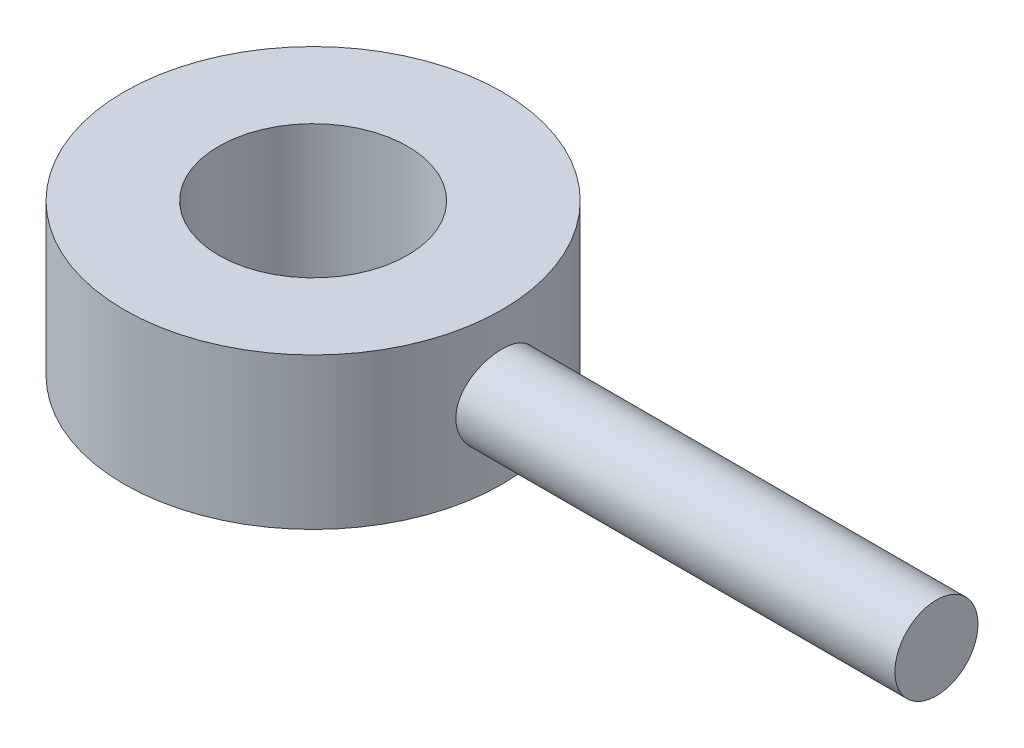
ISO-10303-21;
HEADER;
FILE_DESCRIPTION(('STEP AP214'),'2;1');
FILE_NAME('part.step','',(''),(''),'','','');
FILE_SCHEMA(('AUTOMOTIVE_DESIGN { 1 0 10303 214 1 1 1 1 }'));
ENDSEC;
DATA;
#1=APPLICATION_CONTEXT('core data for automotive mechanical design processes');
#2=APPLICATION_PROTOCOL_DEFINITION('international standard','automotive_design',2000,#1);
#3=PRODUCT_CONTEXT('',#1,'mechanical');
#4=PRODUCT('Part','Part','',(#3));
#5=PRODUCT_RELATED_PRODUCT_CATEGORY('part','',(#4));
#6=PRODUCT_DEFINITION_FORMATION('','',#4);
#7=PRODUCT_DEFINITION_CONTEXT('part definition',#1,'design');
#8=PRODUCT_DEFINITION('design','',#6,#7);
#9=PRODUCT_DEFINITION_SHAPE('','',#8);
#10=(LENGTH_UNIT() NAMED_UNIT(*) SI_UNIT(.MILLI.,.METRE.));
#11=(NAMED_UNIT(*) PLANE_ANGLE_UNIT() SI_UNIT($,.RADIAN.));
#12=(NAMED_UNIT(*) SI_UNIT($,.STERADIAN.) SOLID_ANGLE_UNIT());
#13=UNCERTAINTY_MEASURE_WITH_UNIT(LENGTH_MEASURE(1.E-05),#10,'distance_accuracy_value','');
#14=(GEOMETRIC_REPRESENTATION_CONTEXT(3) GLOBAL_UNCERTAINTY_ASSIGNED_CONTEXT((#13)) GLOBAL_UNIT_ASSIGNED_CONTEXT((#10,
#11,#12)) REPRESENTATION_CONTEXT('',''));
#15=CARTESIAN_POINT('',(0.,0.,0.));
#16=DIRECTION('',(0.,0.,1.));
#17=DIRECTION('',(1.,0.,0.));
#18=AXIS2_PLACEMENT_3D('',#15,#16,#17);
#19=CARTESIAN_POINT('',(0.,4.,0.));
#20=DIRECTION('',(0.,1.,0.));
#21=DIRECTION('',(0.,0.,1.));
#22=AXIS2_PLACEMENT_3D('',#19,#20,#21);
#23=PLANE('',#22);
#24=CARTESIAN_POINT('',(0.,4.,0.));
#25=DIRECTION('',(0.,1.,0.));
#26=DIRECTION('',(0.,0.,1.));
#27=AXIS2_PLACEMENT_3D('',#24,#25,#26);
#28=CIRCLE('',#27,5.);
#29=CARTESIAN_POINT('',(0.,4.,5.));
#30=VERTEX_POINT('',#29);
#31=EDGE_CURVE('E10',#30,#30,#28,.T.);
#32=ORIENTED_EDGE('',*,*,#31,.T.);
#33=EDGE_LOOP('',(#32));
#34=FACE_BOUND('',#33,.T.);
#35=CARTESIAN_POINT('',(0.,4.,0.));
#36=DIRECTION('',(0.,1.,0.));
#37=DIRECTION('',(0.,0.,1.));
#38=AXIS2_PLACEMENT_3D('',#35,#36,#37);
#39=CIRCLE('',#38,2.5);
#40=CARTESIAN_POINT('',(0.,4.,2.5));
#41=VERTEX_POINT('',#40);
#42=EDGE_CURVE('E47',#41,#41,#39,.T.);
#43=ORIENTED_EDGE('',*,*,#42,.F.);
#44=EDGE_LOOP('',(#43));
#45=FACE_BOUND('',#44,.T.);
#46=ADVANCED_FACE('F40',(#34,#45),#23,.T.);
#47=CARTESIAN_POINT('',(0.,0.,0.));
#48=DIRECTION('',(0.,1.,0.));
#49=DIRECTION('',(0.,0.,1.));
#50=AXIS2_PLACEMENT_3D('',#47,#48,#49);
#51=PLANE('',#50);
#52=CARTESIAN_POINT('',(0.,0.,0.));
#53=DIRECTION('',(0.,1.,0.));
#54=DIRECTION('',(0.,0.,1.));
#55=AXIS2_PLACEMENT_3D('',#52,#53,#54);
#56=CIRCLE('',#55,5.);
#57=CARTESIAN_POINT('',(0.,0.,5.));
#58=VERTEX_POINT('',#57);
#59=EDGE_CURVE('E45',#58,#58,#56,.T.);
#60=ORIENTED_EDGE('',*,*,#59,.F.);
#61=EDGE_LOOP('',(#60));
#62=FACE_BOUND('',#61,.T.);
#63=CARTESIAN_POINT('',(0.,0.,0.));
#64=DIRECTION('',(0.,1.,0.));
#65=DIRECTION('',(0.,0.,1.));
#66=AXIS2_PLACEMENT_3D('',#63,#64,#65);
#67=CIRCLE('',#66,2.5);
#68=CARTESIAN_POINT('',(0.,0.,2.5));
#69=VERTEX_POINT('',#68);
#70=EDGE_CURVE('E51',#69,#69,#67,.T.);
#71=ORIENTED_EDGE('',*,*,#70,.T.);
#72=EDGE_LOOP('',(#71));
#73=FACE_BOUND('',#72,.T.);
#74=ADVANCED_FACE('F76',(#62,#73),#51,.F.);
#75=CARTESIAN_POINT('',(0.,4.,0.));
#76=DIRECTION('',(0.,-1.,0.));
#77=DIRECTION('',(0.,0.,-1.));
#78=AXIS2_PLACEMENT_3D('',#75,#76,#77);
#79=CYLINDRICAL_SURFACE('',#78,5.);
#80=CARTESIAN_POINT('',(4.87749935930288,2.,-1.1));
#81=CARTESIAN_POINT('',(4.87750059192786,1.9390201794353,-1.09999791492612));
#82=CARTESIAN_POINT('',(4.87865539644142,1.87801537811326,-1.09491201866376));
#83=CARTESIAN_POINT('',(4.88314122250592,1.75774129032022,-1.07472546298642));
#84=CARTESIAN_POINT('',(4.88647380552498,1.69847328101234,-1.05961761771207));
#85=CARTESIAN_POINT('',(4.89491990534441,1.58342998059707,-1.0198864288525));
#86=CARTESIAN_POINT('',(4.90003145433793,1.52765091028854,-0.995273595944624));
#87=CARTESIAN_POINT('',(4.91145717082736,1.42101230207449,-0.937261257278608));
#88=CARTESIAN_POINT('',(4.91777131651074,1.37015267496603,-0.903861910884835));
#89=CARTESIAN_POINT('',(4.93101133539934,1.27392683949134,-0.828616225712396));
#90=CARTESIAN_POINT('',(4.93794511097895,1.22865694066119,-0.786648093254168));
#91=CARTESIAN_POINT('',(4.95157396934833,1.1457392824436,-0.695719054453303));
#92=CARTESIAN_POINT('',(4.95826903341563,1.10809211983954,-0.646757601115515));
#93=CARTESIAN_POINT('',(4.97075222751559,1.04110713566132,-0.542585501574227));
#94=CARTESIAN_POINT('',(4.97652994590525,1.0118620215218,-0.487313887417924));
#95=CARTESIAN_POINT('',(4.98643815937044,0.963111197150299,-0.372492215823986));
#96=CARTESIAN_POINT('',(4.99056884147107,0.943604381046737,-0.312942645065845));
#97=CARTESIAN_POINT('',(4.99666172270461,0.915187000374263,-0.19225695217033));
#98=CARTESIAN_POINT('',(4.99865724849314,0.906113415539374,-0.131160926699203));
#99=CARTESIAN_POINT('',(5.00037046767797,0.898310289156249,-0.00828344107533812));
#100=CARTESIAN_POINT('',(5.00008842457891,0.899579550986583,0.0534979389590024));
#101=CARTESIAN_POINT('',(4.99730372921666,0.912304833530159,0.174868311810049));
#102=CARTESIAN_POINT('',(4.99483938472223,0.92358512956355,0.234476737170561));
#103=CARTESIAN_POINT('',(4.98801066744812,0.955732158774795,0.350933235851258));
#104=CARTESIAN_POINT('',(4.98364620810345,0.976599328711623,0.40778118327906));
#105=CARTESIAN_POINT('',(4.9734461693194,1.02748268543179,0.517589876653114));
#106=CARTESIAN_POINT('',(4.96759995975693,1.05756532435277,0.570518802020045));
#107=CARTESIAN_POINT('',(4.95507718712354,1.12597609928104,0.670641236268086));
#108=CARTESIAN_POINT('',(4.94840050975635,1.16430537079315,0.717833953910854));
#109=CARTESIAN_POINT('',(4.9347848703112,1.24907752031974,0.806189587464993));
#110=CARTESIAN_POINT('',(4.92784334554032,1.29567418789222,0.847204687115553));
#111=CARTESIAN_POINT('',(4.91461189441242,1.39515617125098,0.920866253616029));
#112=CARTESIAN_POINT('',(4.90832198614041,1.44804166149014,0.953512488233042));
#113=CARTESIAN_POINT('',(4.89709906904939,1.55884098990999,1.00957639469399));
#114=CARTESIAN_POINT('',(4.89217022405119,1.61676956045469,1.03296584029736));
#115=CARTESIAN_POINT('',(4.88428499577542,1.73586913636489,1.06963334728129));
#116=CARTESIAN_POINT('',(4.88132829556883,1.79703961903993,1.08291303337616));
#117=CARTESIAN_POINT('',(4.87778683874614,1.91953517814268,1.09875417213259));
#118=CARTESIAN_POINT('',(4.87715443070833,1.98083105919776,1.10153098432832));
#119=CARTESIAN_POINT('',(4.87820457466623,2.10300992013702,1.09687086480016));
#120=CARTESIAN_POINT('',(4.87988696562385,2.16389292844821,1.08943464358614));
#121=CARTESIAN_POINT('',(4.88533212070861,2.2827660294168,1.0647464744292));
#122=CARTESIAN_POINT('',(4.88906967493981,2.34078207203772,1.04761340088457));
#123=CARTESIAN_POINT('',(4.89818124053484,2.45311998653837,1.00414670243287));
#124=CARTESIAN_POINT('',(4.90355541003142,2.50744150082533,0.977812188429666));
#125=CARTESIAN_POINT('',(4.91543919766926,2.61177959607808,0.91621659031443));
#126=CARTESIAN_POINT('',(4.92196518151733,2.66171604472883,0.880822990698792));
#127=CARTESIAN_POINT('',(4.9353742402688,2.75501980794127,0.802287084126658));
#128=CARTESIAN_POINT('',(4.94225735998362,2.79838629545192,0.759143803103171));
#129=CARTESIAN_POINT('',(4.95576238310321,2.87815643013216,0.665358139823839));
#130=CARTESIAN_POINT('',(4.96237690160789,2.91441316700773,0.614589557453773));
#131=CARTESIAN_POINT('',(4.97446295328537,2.9778834007809,0.507557357883074));
#132=CARTESIAN_POINT('',(4.97993454016225,3.00509732261797,0.451293999053489));
#133=CARTESIAN_POINT('',(4.98908712095463,3.04950552627181,0.335221928140962));
#134=CARTESIAN_POINT('',(4.99277950649837,3.0667636957286,0.275438598062819));
#135=CARTESIAN_POINT('',(4.99800693284399,3.09096976221849,0.153730744771621));
#136=CARTESIAN_POINT('',(4.99954229112212,3.09791917652643,0.0918065380326899));
#137=CARTESIAN_POINT('',(5.0002731072272,3.10124157983504,-0.0310311984112523));
#138=CARTESIAN_POINT('',(4.99951707009963,3.0978338089841,-0.0919386128262422));
#139=CARTESIAN_POINT('',(4.99585410740956,3.08102942125089,-0.212289959032807));
#140=CARTESIAN_POINT('',(4.99294722139187,3.06763298801683,-0.271733917710234));
#141=CARTESIAN_POINT('',(4.9853129244489,3.03133713027188,-0.387299068879444));
#142=CARTESIAN_POINT('',(4.98059153797251,3.00846913363254,-0.443430555354195));
#143=CARTESIAN_POINT('',(4.96983212605049,2.95390980328589,-0.551088880418725));
#144=CARTESIAN_POINT('',(4.96379397121017,2.92221760236689,-0.602615265777603));
#145=CARTESIAN_POINT('',(4.95091484957698,2.85019638228957,-0.700669047552351));
#146=CARTESIAN_POINT('',(4.94406070779334,2.80971338936581,-0.747081628642719));
#147=CARTESIAN_POINT('',(4.93039261746621,2.72156988642554,-0.832529567035146));
#148=CARTESIAN_POINT('',(4.92357867902557,2.67390764598885,-0.871563140639815));
#149=CARTESIAN_POINT('',(4.91065939968106,2.5719811785591,-0.941655472561291));
#150=CARTESIAN_POINT('',(4.90456492229851,2.51763618036073,-0.972598894559436));
#151=CARTESIAN_POINT('',(4.89391152757273,2.40439458465942,-1.02486431597407));
#152=CARTESIAN_POINT('',(4.88935131825545,2.34550186833968,-1.04619441572814));
#153=CARTESIAN_POINT('',(4.88312099991116,2.23879573237756,-1.07484341292603));
#154=CARTESIAN_POINT('',(4.88102694527707,2.19155879645607,-1.08425895070442));
#155=CARTESIAN_POINT('',(4.87821567299023,2.09621972950757,-1.0968379109729));
#156=CARTESIAN_POINT('',(4.87749838666953,2.04811764175183,-1.10000164527932));
#157=CARTESIAN_POINT('',(4.87749935930288,2.,-1.1));
#158=B_SPLINE_CURVE_WITH_KNOTS('',3,(#80,#81,#82,#83,#84,#85,#86,#87,#88,#89,#90,#91,#92,#93,
#94,#95,#96,#97,#98,#99,#100,#101,#102,#103,#104,#105,#106,#107,#108,#109,#110,#111,#112,#113,
#114,#115,#116,#117,#118,#119,#120,#121,#122,#123,#124,#125,#126,#127,#128,#129,#130,#131,#132,
#133,#134,#135,#136,#137,#138,#139,#140,#141,#142,#143,#144,#145,#146,#147,#148,#149,#150,#151,
#152,#153,#154,#155,#156,#157),.UNSPECIFIED.,.T.,.F.,(4,2,2,2,2,2,2,2,2,2,2,2,2,2,2,2,2,2,2,2,2,
2,2,2,2,2,2,2,2,2,2,2,2,2,2,2,2,2,4),(0.,0.182763101090787,0.365657387395347,0.548350004463604,
0.731039308194149,0.91653294157345,1.10204109162356,1.28952374121687,1.47698509561857,
1.66147574685417,1.84594505364379,2.02723901933906,2.20854124524725,2.39118289476655,
2.573849708903,2.76036115186886,2.946877769898,3.13395882042845,3.32100979927812,
3.50420386278735,3.68738518232592,3.86836805363358,4.04936841738637,4.23318501321453,
4.4170247293642,4.60433520453909,4.79163687638516,4.97772283580126,5.16378140378501,
5.34592912523117,5.5280734978526,5.70961827316065,5.89118089635048,6.07622535920624,
6.26131449506935,6.44891386127562,6.6363548563871,6.78057581330699,6.92478957684879),.UNSPECIFIED.);
#159=CARTESIAN_POINT('',(4.87749935930288,2.,-1.1));
#160=VERTEX_POINT('',#159);
#161=EDGE_CURVE('E53',#160,#160,#158,.T.);
#162=ORIENTED_EDGE('',*,*,#161,.T.);
#163=EDGE_LOOP('',(#162));
#164=FACE_BOUND('',#163,.T.);
#165=ORIENTED_EDGE('',*,*,#31,.F.);
#166=EDGE_LOOP('',(#165));
#167=FACE_BOUND('',#166,.T.);
#168=ORIENTED_EDGE('',*,*,#59,.T.);
#169=EDGE_LOOP('',(#168));
#170=FACE_BOUND('',#169,.T.);
#171=ADVANCED_FACE('F39',(#164,#167,#170),#79,.T.);
#172=CARTESIAN_POINT('',(0.,4.,0.));
#173=DIRECTION('',(0.,-1.,0.));
#174=DIRECTION('',(0.,0.,-1.));
#175=AXIS2_PLACEMENT_3D('',#172,#173,#174);
#176=CYLINDRICAL_SURFACE('',#175,2.5);
#177=ORIENTED_EDGE('',*,*,#42,.T.);
#178=EDGE_LOOP('',(#177));
#179=FACE_BOUND('',#178,.T.);
#180=ORIENTED_EDGE('',*,*,#70,.F.);
#181=EDGE_LOOP('',(#180));
#182=FACE_BOUND('',#181,.T.);
#183=ADVANCED_FACE('F69',(#179,#182),#176,.F.);
#184=CARTESIAN_POINT('',(2.5,2.,0.));
#185=DIRECTION('',(1.,0.,0.));
#186=DIRECTION('',(0.,0.,-1.));
#187=AXIS2_PLACEMENT_3D('',#184,#185,#186);
#188=CYLINDRICAL_SURFACE('',#187,1.1);
#189=ORIENTED_EDGE('',*,*,#161,.F.);
#190=EDGE_LOOP('',(#189));
#191=FACE_BOUND('',#190,.T.);
#192=CARTESIAN_POINT('',(16.5,2.,0.));
#193=DIRECTION('',(1.,0.,0.));
#194=DIRECTION('',(0.,0.,-1.));
#195=AXIS2_PLACEMENT_3D('',#192,#193,#194);
#196=CIRCLE('',#195,1.1);
#197=CARTESIAN_POINT('',(16.5,2.,-1.1));
#198=VERTEX_POINT('',#197);
#199=EDGE_CURVE('E62',#198,#198,#196,.T.);
#200=ORIENTED_EDGE('',*,*,#199,.F.);
#201=EDGE_LOOP('',(#200));
#202=FACE_BOUND('',#201,.T.);
#203=ADVANCED_FACE('F63',(#191,#202),#188,.T.);
#204=CARTESIAN_POINT('',(16.5,2.,0.));
#205=DIRECTION('',(1.,0.,0.));
#206=DIRECTION('',(0.,0.,-1.));
#207=AXIS2_PLACEMENT_3D('',#204,#205,#206);
#208=PLANE('',#207);
#209=ORIENTED_EDGE('',*,*,#199,.T.);
#210=EDGE_LOOP('',(#209));
#211=FACE_BOUND('',#210,.T.);
#212=ADVANCED_FACE('F67',(#211),#208,.T.);
#213=CLOSED_SHELL('',(#46,#74,#171,#183,#203,#212));
#214=MANIFOLD_SOLID_BREP('B2',#213);
#215=ADVANCED_BREP_SHAPE_REPRESENTATION('',(#18,#214),#14);
#216=SHAPE_DEFINITION_REPRESENTATION(#9,#215);
ENDSEC;
END-ISO-10303-21;
